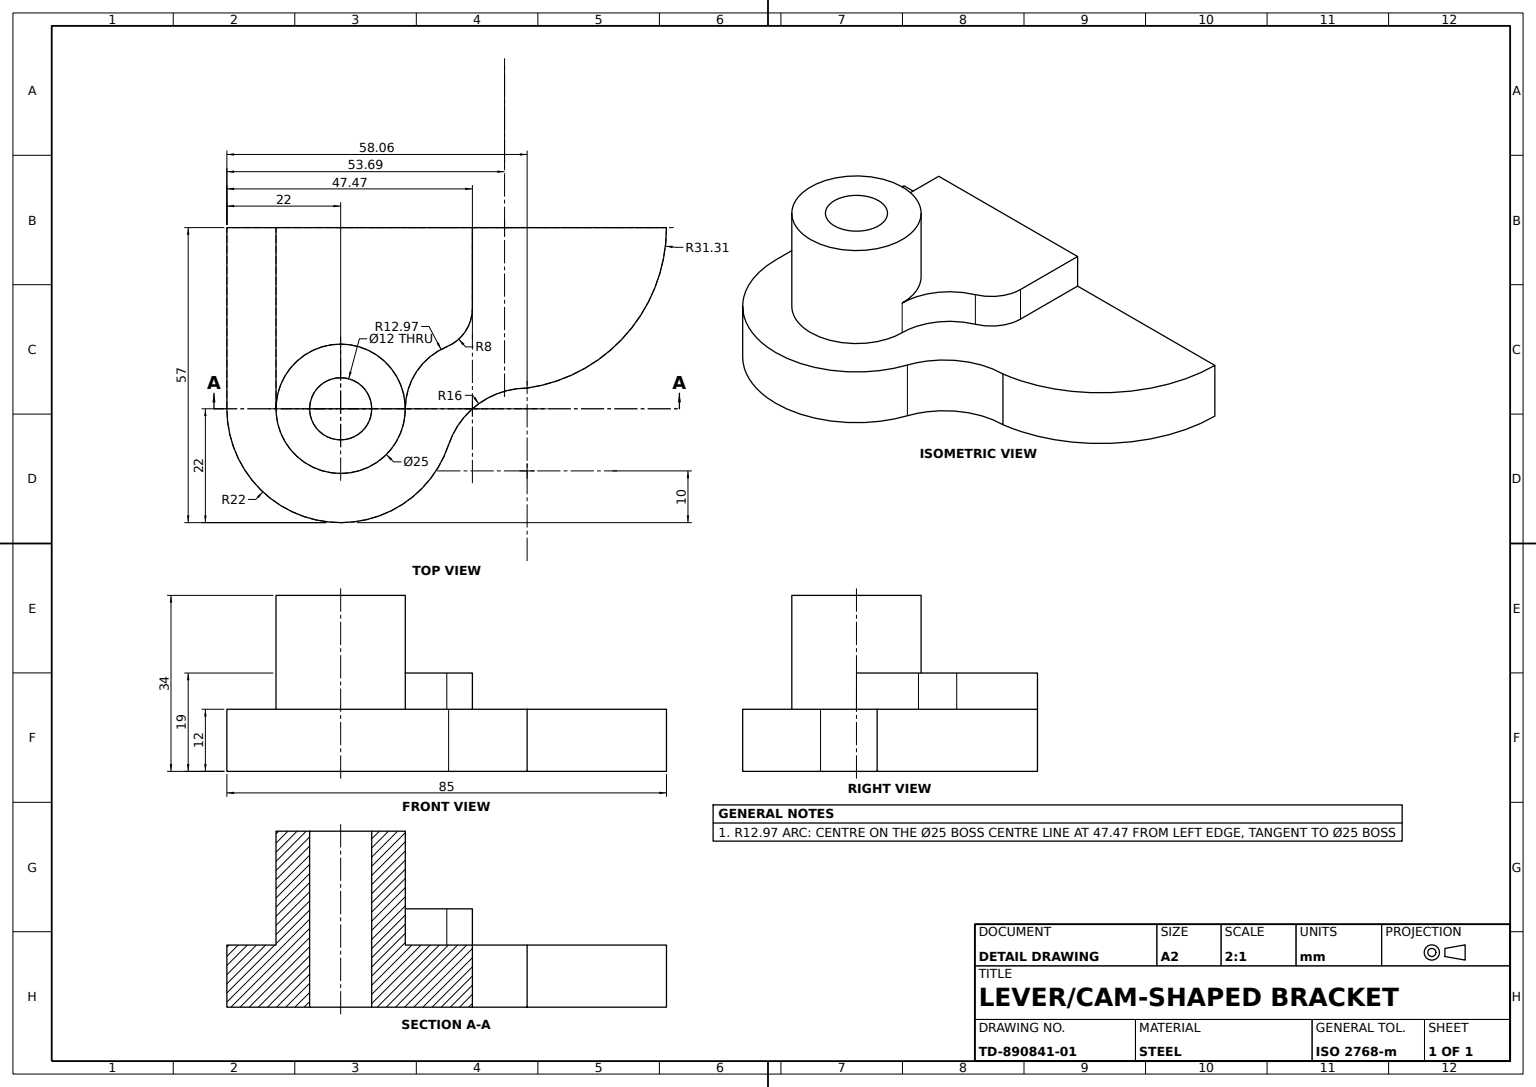
SolidWorks part; units mm, degrees
material "Plain Carbon Steel"
ref_plane "Front Plane" through (0, 0, 0) normal (0, 0, 1) x (1, 0, 0)
ref_plane "Top Plane" through (0, 0, 0) normal (0, 1, 0) x (1, 0, 0)
ref_plane "Right Plane" through (0, 0, 0) normal (1, 0, 0) x (0, 0, -1)
sketch "Base Plate Profile" plane through (0, 0, 0) normal (0, 1, 0) x (1, 0, 0)
  line L1 (-22, 35) -> (63, 35)
  line L2 (-22, 35) -> (-22, 0)
  line L8 (-12.5, 0) -> (-12.5, 35)
  line L9 (-12.5, 35) -> (25.4725, 35)
  line L10 (25.4725, 19.3867) -> (25.4725, 35)
  line L13 (0, 43.7727) -> (0, -38.5195) construction
  line L14 (25.4725, 4) -> (36.0555, 4)
  circle A0 centre (0, 0) radius 12.5
  circle A2 centre (0, 0) radius 6
  arc A3 (36.0555, 4) -> (20.8742, -6.9474) centre (36.0555, -12) ccw
  arc A5 (63, 35) -> (36.0555, 4) centre (31.6948, 35) cw
  arc A7 (-22, 0) -> (20.8742, -6.9474) centre (0, 0) ccw
  arc A8 (20.5241, 11.9916) -> (12.5, 0) centre (25.4725, 0) ccw
  arc A9 (20.5241, 11.9916) -> (25.4725, 19.3867) centre (17.4725, 19.3867) ccw
  point P5 (20.5, 17.5)
  point P6 (36.0555, -12)
  point P10 (6.4863, 17.5)
  point P15 (36.0555, 14.5)
  point P18 (10.9115, -3.6316)
  point P19 (0, 0)
  point P23 (-11.5, 0)
  dimension "D2" = 25
  dimension "D3" = 12
  dimension "D8" = 32
  dimension "D10" = 42.5
  dimension "D13" = 31.3052
  dimension "D9" = 28.4863
  dimension "D12" = 22
  dimension "D4" = 8
  dimension "D5" = 31.3052
  dimension "D6" = 85
  dimension "D7" = 35
  dimension "D11" = 17.5
extrude "Base Plate 12mm" add sketch "Base Plate Profile" along normal blind 12
sketch "Raised Pad Profile" plane through (0, 0, 0) normal (0, 1, 0) x (1, 0, 0)
  line L0 (25.4725, 19.3867) -> (25.4725, 35) construction
  line L1 (-12.5, 0) -> (-12.5, 35) construction
  line L2 (0, 43.7727) -> (0, -38.5195) construction
  line L3 (-22, 35) -> (63, 35) construction
  line L4 (25.4725, 19.3867) -> (25.4725, 35)
  line L5 (63, 35) -> (25.4725, 35)
  line L6 (25.4725, 35) -> (25.4725, 19.3867)
  line L7 (-12.5, 0) -> (-12.5, 35)
  line L8 (-12.5, 35) -> (-22, 35)
  line L9 (-22, 35) -> (-22, 0)
  line L10 (63, 35) -> (25.4725, 35)
  line L11 (25.4725, 35) -> (25.4725, 19.3867)
  line L12 (-12.5, 0) -> (-12.5, 35)
  line L13 (-12.5, 35) -> (-22, 35)
  line L14 (-22, 35) -> (-22, 0)
  line L15 (-12.5, 0) -> (-12.5, 35)
  line L16 (0, 43.7727) -> (0, -38.5195)
  line L17 (-22, 35) -> (63, 35)
  circle A0 centre (0, 0) radius 12.5 construction
  arc A1 (20.5241, 11.9916) -> (25.4725, 19.3867) centre (17.4725, 19.3867) ccw construction
  arc A2 (20.5241, 11.9916) -> (12.5, 0) centre (25.4725, 0) ccw construction
  circle A3 centre (0, 0) radius 6 construction
  circle A4 centre (0, 0) radius 12.5
  arc A5 (20.5241, 11.9916) -> (25.4725, 19.3867) centre (17.4725, 19.3867) ccw
  arc A6 (36.0555, 4) -> (20.8742, -6.9474) centre (36.0555, -12) ccw
  arc A7 (36.0555, 4) -> (63, 35) centre (31.6948, 35) ccw
  arc A8 (20.5241, 11.9916) -> (25.4725, 19.3867) centre (17.4725, 19.3867) ccw
  arc A9 (20.5241, 11.9916) -> (12.5, 0) centre (25.4725, 0) ccw
  arc A10 (-12.5, 0) -> (12.5, 0) centre (0, 0) ccw
  arc A11 (-22, 0) -> (20.8742, -6.9474) centre (0, 0) ccw
  arc A12 (36.0555, 4) -> (20.8742, -6.9474) centre (36.0555, -12) ccw
  arc A13 (36.0555, 4) -> (63, 35) centre (31.6948, 35) ccw
  arc A14 (20.5241, 11.9916) -> (25.4725, 19.3867) centre (17.4725, 19.3867) ccw
  arc A15 (20.5241, 11.9916) -> (12.5, 0) centre (25.4725, 0) ccw
  arc A16 (-12.5, 0) -> (12.5, 0) centre (0, 0) ccw
  arc A17 (-22, 0) -> (20.8742, -6.9474) centre (0, 0) ccw
  arc A18 (20.5241, 11.9916) -> (12.5, 0) centre (25.4725, 0) ccw
  circle A19 centre (0, 0) radius 6
  dimension "D1" = 0
extrude "Raised Pad 19mm" add sketch "Raised Pad Profile" along normal blind 19 contours A15 A5 L4 L17 L16 A4 | A4 L16 L17 L12
sketch "Hub Profile" plane through (0, 0, 0) normal (0, 1, 0) x (1, 0, 0)
  circle A0 centre (0, 0) radius 12.5 construction
  circle A1 centre (0, 0) radius 12.5
  circle A2 centre (0, 0) radius 6 construction
  circle A3 centre (0, 0) radius 6
extrude "Hub Boss 34mm" add sketch "Hub Profile" along normal blind 34
